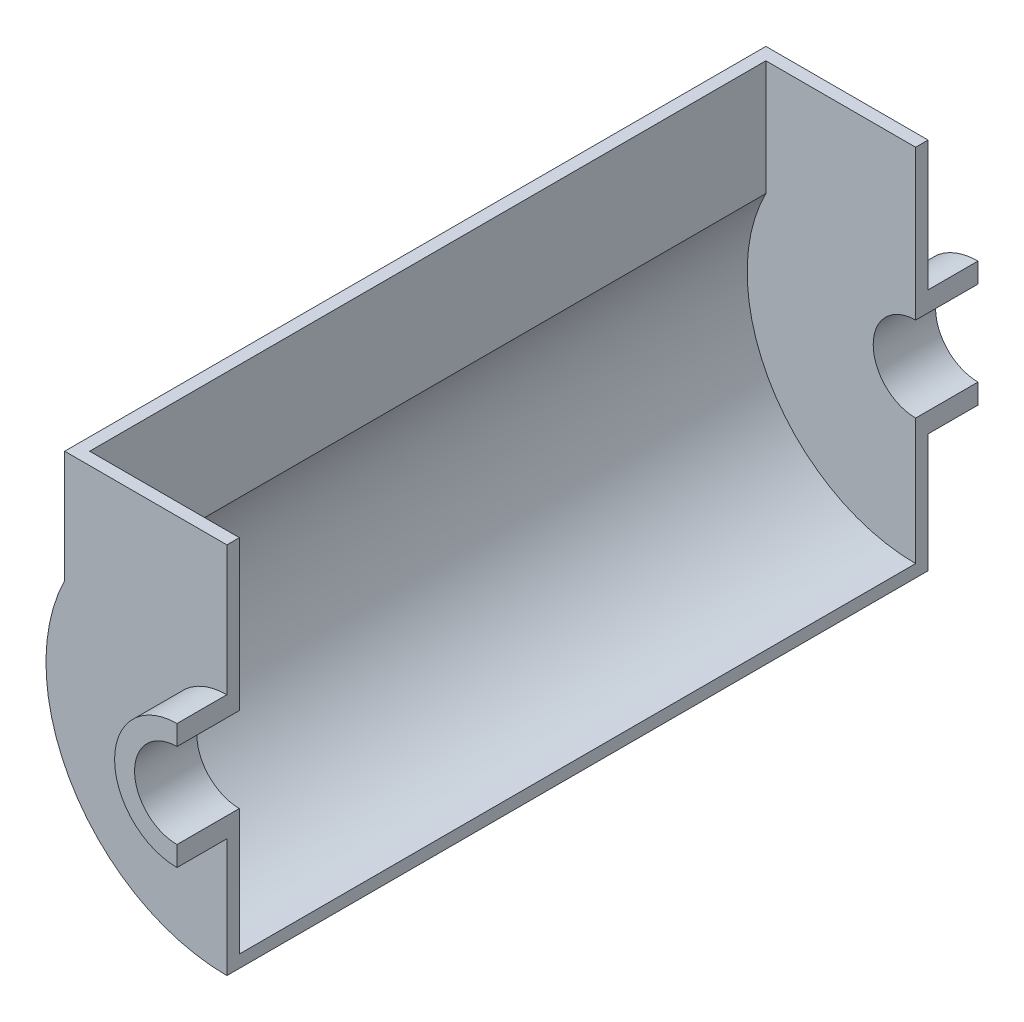
from build123d import *

# Parameters (mm, degrees)
TROUGH_SHELL_DEPTH      = 20
TROUGH_SHELL_DEPTH_BACK = 5
END_START               = -5
END_PLATE_DEPTH         = 5
SIDE_WALLS_REACH        = 316.327


with BuildPart() as part:
    # Trough Profile Sketch → Trough Shell (new, two sides: drawn at the far end of the back side and taken through both)
    with BuildSketch(Plane.XY.offset(-TROUGH_SHELL_DEPTH_BACK)):
        with BuildLine():
            Line((0, 17), (0, 25))
            ThreePointArc((0, 25), (-25, 0), (0, -25))
            Line((0, -25), (0, -17))
            ThreePointArc((0, -17), (-17, 0), (0, 17))
        make_face()
    extrude(amount=TROUGH_SHELL_DEPTH + TROUGH_SHELL_DEPTH_BACK)

    # End Plate Sketch → End Plate (add)
    with BuildSketch(Plane.XY.offset(END_START)):
        with BuildLine():
            Line((0, 25), (0, 77))
            Line((0, 77), (-65, 77))
            Line((-65, 77), (-65, 32.113081447))
            ThreePointArc((-65, 32.113081447), (-61.581037686, -38.262590053), (0, -72.5))
            Line((0, -72.5), (0, -25))
            ThreePointArc((0, -25), (-25, 0), (0, 25))
        make_face()
    extrude(amount=END_PLATE_DEPTH)


with BuildPart() as body_2:
    # End Plate Mirror: mirrored copy
    add(part.part.mirror(Plane.XY.offset(-140.5)))

    # Side Wall Sketch → Side Walls (add, up to next)
    with BuildSketch(Plane(origin=(0, 0, -5), x_dir=(-1, 0, 0), z_dir=(0, 0, -1)), mode=Mode.PRIVATE) as side_walls_sk1:
        with BuildLine():
            Line((65, 77), (65, 32.113081447))
            ThreePointArc((65, 32.113081447), (61.581037686, -38.262590053), (0, -72.5))
            Line((0, -72.5), (0, -67.5))
            ThreePointArc((0, -67.5), (57.634938288, -35.134938288), (60, 30.923292192))
            Line((60, 30.923292192), (60, 77))
            Line((60, 77), (65, 77))
        make_face()
    side_walls_tool1 = extrude(side_walls_sk1.sketch, amount=SIDE_WALLS_REACH, mode=Mode.PRIVATE) - body_2.part

    add(part.part)  # Side Walls merges part
    add(side_walls_tool1.solids().sort_by_distance((-61.66152, 53.961646, -5))[0])


solid = body_2.part
